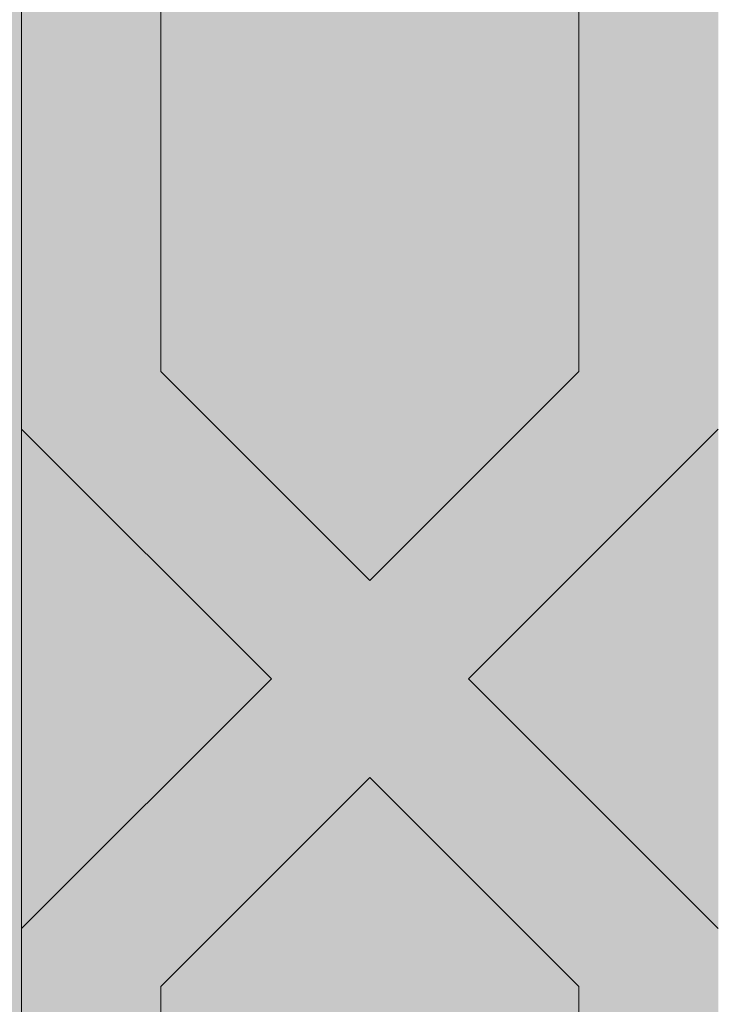
# Model space of a CAD drawing. Units: inches. Extents: x 844 to 2234, y 346 to 1084.
# Tile 70 of 93: x 1997.478 to 1998.757, y 692.525 to 694.327. Entities that reach past the tile are written whole.
import ezdxf

# ---------------------------------------------------------------- set-up
doc = ezdxf.new("R2010")
doc.units = ezdxf.units.IN
doc.header["$MEASUREMENT"] = 0
for name, color, linetype, lineweight in [('A-ANNO-DIMS', 2, 'Continuous', 18), ('furniture', 8, 'Continuous', 18), ('RA-AP-01$0$INT', 35, 'Continuous', 5)]:
    doc.layers.add(name, color=color, linetype=linetype, lineweight=lineweight)
doc.layers.add('RA-AP-01$0$FURN', color=3, linetype='Continuous')
doc.styles.get("Standard").update_dxf_attribs({"font": 'arial.ttf'})
doc.dimstyles.get("Standard").update_dxf_attribs({"dimtxt": 6, "dimasz": 3, "dimexe": 0.18, "dimexo": 0.0625, "dimgap": 0.09, "dimtad": 0, "dimtih": 1, "dimtoh": 1, "dimdec": 1, "dimzin": 0, "dimdsep": 46, "dimlunit": 3, "dimtxsty": 'Standard', "dimblk": 'ARCHTICK', "dimcen": 0.09, "dimadec": 0, "dimazin": 0, "dimtfac": 1, "dimtdec": 1, "dimtofl": 0, "dimtmove": 0, "dimatfit": 3, "dimfxl": 1, "dimtolj": 1, "dimtzin": 0, "dimarcsym": 0})

# ---------------------------------------------------------------- blocks, each defined once
blk = doc.blocks.new('A$C18D01794')
at = {"layer": 'RA-AP-01$0$INT'}
h = blk.add_hatch(color=256, dxfattribs=at)
h.paths.add_polyline_path([(4.355206456958071, -6.156712009588037), (4.355206456958071, -8.056712009588038), (5.455206456958072, -8.056712009588038), (5.455206456958072, -6.156712009588037)])
h.paths.add_polyline_path([(4.405206456958072, -8.006712009588039), (4.405206456958072, -6.206712009588038), (5.405206456958072, -6.206712009588038), (5.405206456958072, -8.006712009588039)], flags=16)
h = blk.add_hatch(color=256, dxfattribs=at)
h.paths.add_polyline_path([(4.469348592586677, -7.07085414521094), (4.505206456958073, -7.03499628085108), (4.505206456958071, -7.106712009593861)])
h.paths.add_polyline_path([(4.455206456960671, -7.084996280832395), (4.476922185709333, -7.106712009588038), (4.433490728198045, -7.106712009588038)])
h.paths.add_polyline_path([(4.405206456958073, -7.034996280813718), (4.441064321339218, -7.070854145206393), (4.40520645695807, -7.106712009576003)])
h.paths.add_polyline_path([(4.425206456989053, -6.911460746921742), (4.455206456990736, -6.881460746929706), (4.485206456989055, -6.911460746937677), (4.48520645696979, -7.026712009590022), (4.455206456965227, -7.056712009584936), (4.425206456969784, -7.026712009579853)])
h.paths.add_polyline_path([(4.505206456958073, -6.831460746955388), (4.505206456958071, -6.903176475661116), (4.469348592616738, -6.867318611308251)])
h.paths.add_polyline_path([(4.425206456964688, -6.707925213036777), (4.455206456964794, -6.677925213027025), (4.485206456964689, -6.707925213017265), (4.485206456983951, -6.823176475683938), (4.455206456990736, -6.853176475686799), (4.425206456983956, -6.823176475689667)])
h.paths.add_polyline_path([(4.425206456974126, -6.504389679118949), (4.455206456959092, -6.474389679124341), (4.485206456974132, -6.504389679129721), (4.485206456993396, -6.619640941768059), (4.45520645699153, -6.649640941779566), (4.425206456993394, -6.619640941791077)])
h.paths.add_polyline_path([(4.46934859260189, -6.663783077416661), (4.505206456958071, -6.627925213048953), (4.505206456958073, -6.699640941761311)])
h.paths.add_polyline_path([(4.405206456958073, -6.627925213005104), (4.441064321354427, -6.663783077389926), (4.405206456958072, -6.699640941797813)])
h.paths.add_polyline_path([(4.405206456958072, -6.424389679139403), (4.441064321333084, -6.460247543502882), (4.405206456958072, -6.496105407889427)])
h.paths.add_polyline_path([(4.469348592580547, -6.460247543498336), (4.505206456958071, -6.424389679109282), (4.505206456958071, -6.496105407864332)])
h.paths.add_polyline_path([(4.425206456957888, -6.300854145208262), (4.45520645695415, -6.270854145221655), (4.485206456959507, -6.300854145217359), (4.48520645695824, -6.416105407863534), (4.455206456954537, -6.44610540787688), (4.425206456957888, -6.416105407889874)])
h.paths.add_polyline_path([(4.425206456957888, -6.226712009591025), (4.471064321332215, -6.226712009591025), (4.425206456957888, -6.272569873980103)])
h.paths.add_polyline_path([(4.499348592575121, -6.226712009591029), (4.636064321343707, -6.226712009591025), (4.666064321342317, -6.256712009589254), (4.636064321340932, -6.286712009591028), (4.499348592588945, -6.286712009591028), (4.469348592591685, -6.256712009584116)])
h.paths.add_polyline_path([(4.680206456964641, -6.270854145214393), (4.716064321337824, -6.306712009588038), (4.644348592591454, -6.306712009588038)])
h.paths.add_polyline_path([(4.644348592588108, -6.206712009588038), (4.716064321341167, -6.206712009588038), (4.680206456964637, -6.242569873964111)])
h.paths.add_polyline_path([(4.724348592586768, -6.226712009589824), (4.861064321340514, -6.226712009589824), (4.891064321340324, -6.256712009589255), (4.861064321340141, -6.286712009589827), (4.724348592587134, -6.286712009589821), (4.694348592586957, -6.256712009589254)])
h.paths.add_polyline_path([(4.905206456964143, -6.270854145212892), (4.941064321338827, -6.306712009588038), (4.869348592589457, -6.306712009588039)])
h.paths.add_polyline_path([(4.869348592586113, -6.206712009588038), (4.941064321342172, -6.206712009588038), (4.905206456964145, -6.242569873965612)])
h.paths.add_polyline_path([(4.949348592587774, -6.226712009589824), (5.086064321341521, -6.226712009589824), (5.116064321341329, -6.256712009589252), (5.08606432134115, -6.286712009589823), (4.949348592588145, -6.286712009589827), (4.919348592587961, -6.256712009589255)])
h.paths.add_polyline_path([(5.130206456963645, -6.270854145214393), (5.166064321336834, -6.306712009588038), (5.094348592590464, -6.306712009588038)])
h.paths.add_polyline_path([(5.094348592587119, -6.206712009588038), (5.166064321340178, -6.206712009588038), (5.130206456963651, -6.242569873964107)])
h.paths.add_polyline_path([(5.174348592584578, -6.226712009591027), (5.311064321353163, -6.226712009591027), (5.341064321336602, -6.256712009584116), (5.31106432133934, -6.286712009591028), (5.174348592587352, -6.286712009591028), (5.144348592585969, -6.256712009589254)])
h.paths.add_polyline_path([(5.325206456968778, -6.300854145217359), (5.355206456974136, -6.270854145221653), (5.385206456970396, -6.300854145208262), (5.385206456970396, -6.416105407889878), (5.355206456973747, -6.44610540787688), (5.325206456970044, -6.416105407863533)])
h.paths.add_polyline_path([(5.339348592596073, -6.226712009591029), (5.385206456970396, -6.226712009591025), (5.385206456970398, -6.272569873980105)])
h.paths.add_polyline_path([(5.325206456954155, -6.504389679129722), (5.355206456969194, -6.474389679124342), (5.38520645695416, -6.504389679118949), (5.385206456934896, -6.619640941791077), (5.355206456936758, -6.649640941779564), (5.325206456934888, -6.619640941768057)])
h.paths.add_polyline_path([(5.305206456958072, -6.424389679097139), (5.341064321347739, -6.460247543498338), (5.305206456958072, -6.496105407876472)])
h.paths.add_polyline_path([(5.369348592595204, -6.460247543502882), (5.40520645695807, -6.42438967915155), (5.405206456958072, -6.496105407877278)])
h.paths.add_polyline_path([(5.405206456958072, -6.627925213017245), (5.405206456958072, -6.69964094178567), (5.369348592573857, -6.663783077389926)])
h.paths.add_polyline_path([(5.305206456958072, -6.62792521303681), (5.341064321326393, -6.663783077416663), (5.305206456958072, -6.69964094177345)])
h.paths.add_polyline_path([(5.325206456963599, -6.707925213017267), (5.355206456963494, -6.677925213027021), (5.385206456963598, -6.707925213036775), (5.385206456944334, -6.823176475689665), (5.355206456937552, -6.853176475686797), (5.325206456944333, -6.823176475683936)])
h.paths.add_polyline_path([(5.305206456958072, -6.831460746943246), (5.341064321311551, -6.867318611308252), (5.305206456958072, -6.903176475673257)])
h.paths.add_polyline_path([(5.325206456939231, -6.911460746937672), (5.355206456937552, -6.881460746929707), (5.385206456939235, -6.911460746921742), (5.385206456958502, -7.026712009579853), (5.355206456963061, -7.056712009584934), (5.3252064569585, -7.026712009590026)])
h.paths.add_polyline_path([(5.404581768715993, -6.832085435167151, 0.001217816984214), (5.405206456958072, -6.832312009593747), (5.405206456958072, -6.90317647569123), (5.369348592563558, -6.867318611308251)])
h.paths.add_polyline_path([(5.36934859258907, -7.070854145206393), (5.40520645695807, -7.034996280825861), (5.405206456958072, -7.106712009563858)])
h.paths.add_polyline_path([(5.355206456967613, -7.084996280832394), (5.376922185730239, -7.106712009588038), (5.333490728218953, -7.106712009588036)])
h.paths.add_polyline_path([(5.30520645695807, -7.034996280838937), (5.341064321341609, -7.070854145210942), (5.305206456958074, -7.106712009606006)])
h = blk.add_hatch(color=256, dxfattribs=at)
h.paths.add_polyline_path([(4.505206456958071, -6.627925213048953), (4.46934859260189, -6.663783077416663), (4.505206456958071, -6.699640941761309), (4.505206456958071, -6.831460746955389), (4.469348592616735, -6.867318611308252), (4.505206456958071, -6.903176475661112), (4.505206456958071, -7.03499628085108), (4.469348592586679, -7.070854145210939), (4.505206456952245, -7.106712009588038), (4.476922185709333, -7.106712009588038), (4.455206456960671, -7.084996280832395), (4.433490728198047, -7.106712009588038), (4.405206456946033, -7.10671200958804), (4.441064321339216, -7.070854145206393), (4.40520645695807, -7.034996280813718), (4.405206456958072, -6.903176475703379), (4.441064321364728, -6.867318611308251), (4.40520645695807, -6.83146074691313), (4.40520645695807, -6.699640941797813), (4.441064321354429, -6.663783077389924), (4.405206456958072, -6.627925213005102), (4.405206456958072, -6.496105407889425), (4.441064321333084, -6.460247543502882), (4.405206456958072, -6.424389679139403), (4.405206456958072, -6.206712009588038), (4.644348592588106, -6.206712009588038), (4.680206456964639, -6.242569873964107), (4.716064321341165, -6.206712009588038), (4.869348592586113, -6.206712009588038), (4.905206456964143, -6.24256987396561), (4.941064321342174, -6.206712009588038), (5.094348592587118, -6.206712009588038), (5.130206456963649, -6.242569873964107), (5.166064321340178, -6.206712009588038), (5.405206456958072, -6.206712009588038), (5.405206456958072, -6.42438967915155), (5.369348592595202, -6.46024754350288), (5.40520645695807, -6.49610540787728), (5.40520645695807, -6.627925213017247), (5.369348592573859, -6.663783077389926), (5.40520645695807, -6.699640941785666), (5.40520645695807, -6.831460746925273), (5.36934859256356, -6.867318611308252), (5.405206456958072, -6.90317647569123), (5.405206456958072, -7.034996280825859), (5.369348592589068, -7.070854145206395), (5.405206456982249, -7.106712009588038), (5.376922185730244, -7.106712009588038), (5.355206456967613, -7.084996280832397), (5.333490728218955, -7.106712009588036), (5.305206456976043, -7.106712009588035), (5.341064321341609, -7.07085414521094), (5.305206456958072, -7.034996280838935), (5.305206456958072, -6.90317647567326), (5.34106432131155, -6.867318611308252), (5.305206456958072, -6.831460746943244), (5.30520645695807, -6.699640941773452), (5.341064321326395, -6.663783077416663), (5.305206456958072, -6.627925213036814), (5.305206456958072, -6.496105407876472), (5.341064321347738, -6.46024754349834), (5.305206456958072, -6.424389679097137), (5.30520645695807, -6.306712009588038), (5.166064321336834, -6.306712009588038), (5.130206456963647, -6.270854145214393), (5.094348592590464, -6.306712009588038), (4.941064321338827, -6.306712009588036), (4.905206456964145, -6.270854145212892), (4.869348592589459, -6.306712009588038), (4.716064321337822, -6.306712009588036), (4.680206456964641, -6.270854145214393), (4.644348592591453, -6.306712009588038), (4.505206456958071, -6.306712009588038), (4.505206456958071, -6.424389679109282), (4.469348592580545, -6.460247543498338), (4.505206456958071, -6.496105407864328)])
h.paths.add_polyline_path([(4.485206456974132, -6.504389679129722), (4.45520645695909, -6.474389679124341), (4.425206456974128, -6.504389679118945), (4.425206456993394, -6.619640941791079), (4.45520645699153, -6.649640941779566), (4.485206456993396, -6.619640941768059)], flags=16)
h.paths.add_polyline_path([(4.455206456954537, -6.44610540787688), (4.485206456958242, -6.416105407863534), (4.48520645695951, -6.30085414521736), (4.45520645695415, -6.270854145221653), (4.425206456957888, -6.300854145208264), (4.425206456957888, -6.41610540788988)], flags=16)
h.paths.add_polyline_path([(4.455206456964794, -6.677925213027025), (4.42520645696469, -6.707925213036777), (4.425206456983954, -6.82317647568967), (4.455206456990734, -6.853176475686797), (4.485206456983953, -6.823176475683936), (4.485206456964687, -6.707925213017265)], flags=16)
h.paths.add_polyline_path([(4.499348592588947, -6.286712009591028), (4.636064321340932, -6.286712009591028), (4.666064321342317, -6.256712009589254), (4.636064321343707, -6.226712009591027), (4.499348592575121, -6.226712009591029), (4.469348592591685, -6.256712009584118)], flags=16)
h.paths.add_polyline_path([(4.425206456957888, -6.272569873980103), (4.471064321332215, -6.226712009591025), (4.425206456957888, -6.226712009591025)], flags=16)
h.paths.add_polyline_path([(4.455206456990734, -6.881460746929709), (4.425206456989053, -6.91146074692174), (4.425206456969784, -7.026712009579853), (4.455206456965226, -7.056712009584932), (4.485206456969787, -7.026712009590026), (4.485206456989053, -6.911460746937672)], flags=16)
h.paths.add_polyline_path([(4.72434859258714, -6.286712009589821), (4.861064321340141, -6.286712009589829), (4.891064321340324, -6.256712009589254), (4.861064321340513, -6.226712009589823), (4.724348592586768, -6.226712009589823), (4.694348592586956, -6.256712009589254)], flags=16)
h.paths.add_polyline_path([(4.919348592587961, -6.256712009589254), (4.949348592588145, -6.286712009589827), (5.08606432134115, -6.286712009589823), (5.116064321341327, -6.256712009589254), (5.086064321341519, -6.226712009589824), (4.949348592587774, -6.226712009589824)], flags=16)
h.paths.add_polyline_path([(5.144348592585967, -6.256712009589254), (5.174348592587358, -6.286712009591028), (5.311064321339338, -6.286712009591028), (5.3410643213366, -6.256712009584118), (5.311064321353163, -6.226712009591029), (5.174348592584576, -6.226712009591027)], flags=16)
h.paths.add_polyline_path([(5.32520645693489, -6.619640941768055), (5.355206456936755, -6.649640941779566), (5.385206456934894, -6.619640941791079), (5.38520645695416, -6.504389679118949), (5.355206456969194, -6.474389679124341), (5.325206456954153, -6.504389679129724)], flags=16)
h.paths.add_polyline_path([(5.325206456970042, -6.416105407863534), (5.355206456973747, -6.44610540787688), (5.385206456970398, -6.416105407889876), (5.385206456970398, -6.30085414520826), (5.355206456974136, -6.270854145221653), (5.325206456968778, -6.30085414521736)], flags=16)
h.paths.add_polyline_path([(5.325206456963599, -6.707925213017265), (5.325206456944333, -6.823176475683936), (5.355206456937552, -6.853176475686797), (5.385206456944332, -6.823176475689667), (5.385206456963596, -6.707925213036773), (5.355206456963492, -6.677925213027027)], flags=16)
h.paths.add_polyline_path([(5.32520645693923, -6.911460746937674), (5.3252064569585, -7.026712009590026), (5.355206456963062, -7.056712009584934), (5.3852064569585, -7.026712009579853), (5.385206456939234, -6.911460746921738), (5.355206456937552, -6.881460746929707)], flags=16)
h.paths.add_polyline_path([(5.339348592596071, -6.226712009591029), (5.385206456970398, -6.272569873980103), (5.385206456970396, -6.226712009591027)], flags=16)
for p, q in [((5.325206456968778, -6.300854145217359), (5.325206456970044, -6.416105407863533)), ((5.385206456970398, -6.416105407889878), (5.385206456970398, -6.300854145208262)), ((5.355206456973749, -6.44610540787688), (5.325206456970044, -6.416105407863533)), ((5.355206456973749, -6.44610540787688), (5.385206456970398, -6.416105407889878)), ((5.341064321347739, -6.460247543498338), (5.305206456976345, -6.424389679115412)), ((5.369348592595202, -6.460247543502882), (5.40520645697813, -6.42438967913149)), ((5.305206456965273, -6.49610540786927), (5.341064321347739, -6.460247543498338)), ((5.405206456965273, -6.496105407884483), (5.369348592595202, -6.460247543502882)), ((5.325206456954155, -6.504389679129722), (5.355206456969194, -6.474389679124341)), ((5.385206456954159, -6.504389679118947), (5.355206456969194, -6.474389679124341)), ((5.32520645693489, -6.619640941768059), (5.325206456954155, -6.504389679129722)), ((5.385206456934892, -6.619640941791081), (5.385206456954159, -6.504389679118947))]:
    blk.add_line(p, q, dxfattribs=at)
blk.add_lwpolyline([(5.405206456958072, -7.106712009588038), (5.405206456958072, -6.206712009588038)], dxfattribs=at)
blk = doc.blocks.new('A$C5D2F253E')
at = {"layer": 'RA-AP-01$0$FURN', "xscale": -0.7999999999883585, "yscale": 0.7999999999883585, "zscale": 0.8, "rotation": 90}
blk.add_blockref('A$C18D01794', (-5.687757199772477, 4.75791982714071), dxfattribs=at)
blk = doc.blocks.new('_ArchTick')
at = {"color": 0, "linetype": 'ByBlock', "const_width": 0.15}
blk.add_lwpolyline([(-0.5, -0.5), (0.5, 0.5)], dxfattribs=at)
blk = doc.blocks.new('*D121')
at = {"layer": 'A-ANNO-DIMS', "color": 0, "lineweight": -2, "transparency": 16777216}
for p, q in [((2030.271987351997, 734.262611118704), (2040.245275089302, 734.262611118704)), ((2040.065275089302, 734.262611118704), (2040.065275089302, 704.6043509484256)), ((2040.065275089302, 668.557359536674), (2040.065275089302, 698.2156197069523)), ((2030.271987351997, 668.557359536674), (2040.245275089302, 668.557359536674))]:
    blk.add_line(p, q, dxfattribs=at)
at = {"layer": 'Defpoints', "color": 0, "transparency": 16777216}
for p in [(2030.209487351997, 734.262611118704), (2040.065275089302, 734.262611118704), (2030.209487351997, 668.557359536674)]:
    blk.add_point(p, dxfattribs=at)
at = {"layer": 'A-ANNO-DIMS', "color": 0, "lineweight": -2, "transparency": 16777216, "xscale": 3, "yscale": 3, "zscale": 3}
for p, rotation in [((2040.065275089302, 734.262611118704), 90), ((2040.065275089302, 668.557359536674), 270)]:
    blk.add_blockref('_ArchTick', p, dxfattribs=dict(at, rotation=rotation))
at = {"layer": 'A-ANNO-DIMS', "color": 0, "transparency": 16777216, "insert": (2040.065275089302, 701.4099853276883), "char_height": 6, "attachment_point": 5}
blk.add_mtext('\\A1;LOUNGE SET 5\'-5 1/2" TYP.', dxfattribs=at)

msp = doc.modelspace()

# ---------------------------------------------------------------- block references
at = {"layer": 'furniture', "xscale": -15.94108302203742, "yscale": 15.94108302203742, "zscale": 15.94108302203742, "rotation": 270}
msp.add_blockref('A$C5D2F253E', (1990.567271852805, 701.4028671565849), dxfattribs=at)

# ---------------------------------------------------------------- dimensions: what is measured, and where the dimension line sits
at = {"layer": 'A-ANNO-DIMS'}
dim = msp.add_linear_dim(base=(2040.065275089302, 734.262611118704), p1=(2030.209487351996, 668.5573595366737), p2=(2030.209487351996, 734.2626111187037), angle=90, text='LOUNGE SET <> TYP.', dimstyle='Standard', override={"dimdec": 1, "dimlfac": 1, "dimrnd": 0, "dimzin": 1, "dimdsep": 46, "dimlunit": 4, "dimfrac": 2}, dxfattribs=at)
dim.commit()
dim.dimension.update_dxf_attribs({"geometry": '*D121', "text_midpoint": (2040.065275089302, 701.4099853276883)})

doc.saveas('drawing.dxf')
